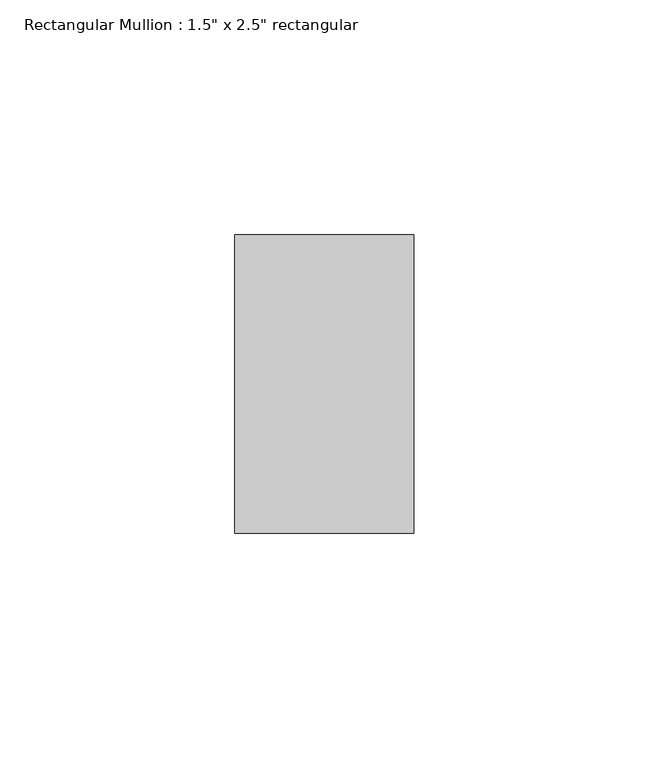
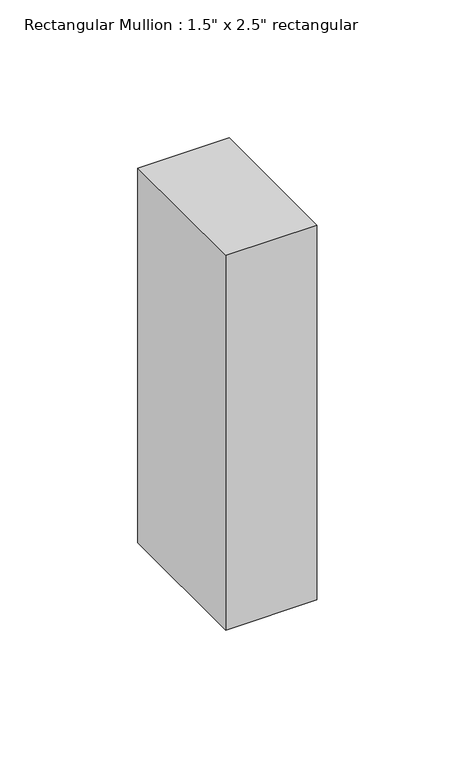
"""IFC4 building model written with IfcOpenShell, lengths in millimetres: member geometry."""

from ifc_helpers import new_model, si_unit, frame, origin, place, context, project, spatial, polyline, outline, extrude, source, transform, mapped, element, save


def member_a59c64b1(model_context):
    return source(origin(), model_context, "Body", "SweptSolid", [
        extrude(outline(polyline([(19.05, 31.75), (19.05, -31.75), (-19.05, -31.75), (-19.05, 31.75), (19.05, 31.75)])), frame((0.0, 0.0, -165.7826151), z_axis=(0.0, 0.0, 1.0), x_axis=(1.0, 0.0, 0.0)), (0.0, 0.0, 1.0), 165.7826151),
    ])


if __name__ == "__main__":
    model = new_model("IFC4")
    model_context = context("Model", 3, world=origin())
    ifc_project = project(units=[si_unit("LENGTHUNIT", "METRE", prefix="MILLI")], contexts=[model_context])
    site = spatial("IfcSite", under=ifc_project)
    building = spatial("IfcBuilding", under=site)
    placement = place(None, origin())
    member_shape = member_a59c64b1(model_context)
    element("IfcMember", 1, ObjectType="Rectangular Mullion : 1.5\" x 2.5\" rectangular", at=placement, inside=building, context=model_context, shape_type="MappedRepresentation", body=[
        mapped(member_shape, transform((0.0, 0.0, 0.0), x_axis=(1.0, 0.0, 0.0), y_axis=(0.0, 1.0, 0.0), z_axis=(0.0, 0.0, 1.0))),
    ])
    save(model, "model.ifc")

# Revit data of these elements
# Type "Rectangular Mullion : 1.5\" x 2.5\" rectangular"
#   built-in parameter 1007304 = 0.208333 (stored number, unit not read)
#   built-in parameter 1007301 = 0.0625 (stored number, unit not read)
#   built-in parameter 1007300 = 0.0625 (stored number, unit not read)
# Element 1 (IfcMember, "Rectangular Mullion : 1.5\" x 2.5\" rectangular")
#   Materials on its faces: "Aluminum"
# Materials
#   "Aluminum": class "Metal", colour RGB 247 247 247, transparency 0, Description = "Aluminum 6061", Cost = 0
